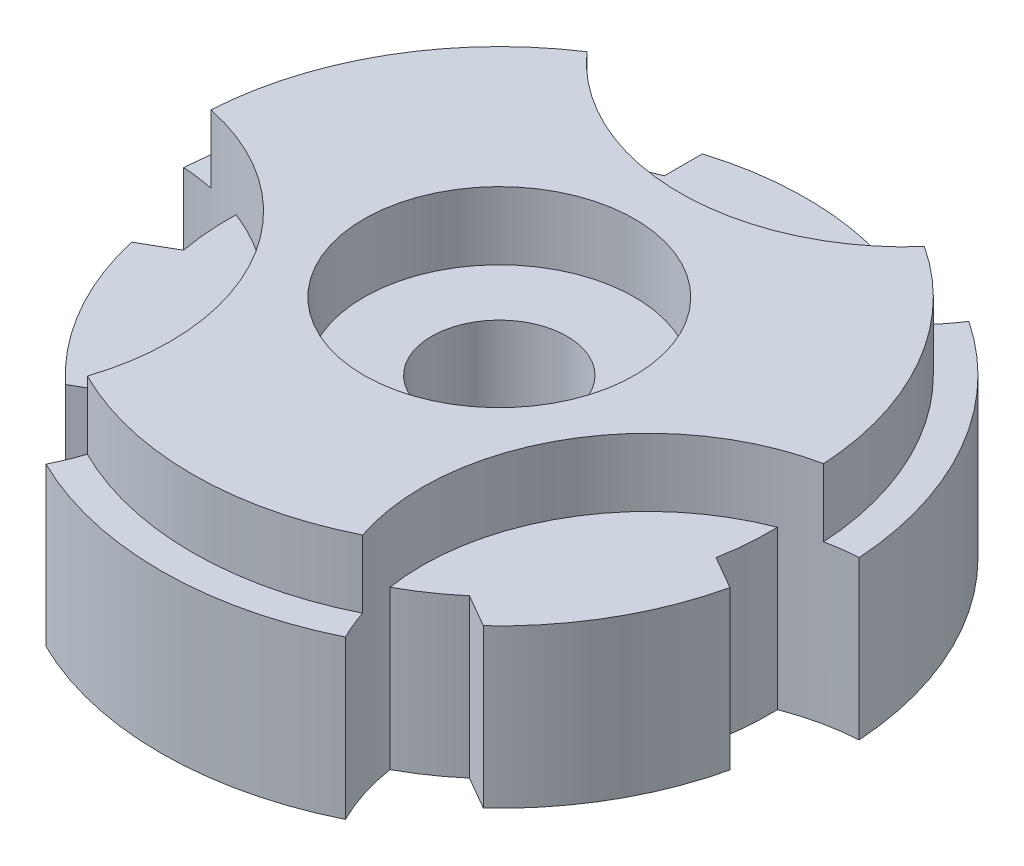
ISO-10303-21;
HEADER;
FILE_DESCRIPTION(('STEP AP214'),'2;1');
FILE_NAME('part.step','',(''),(''),'','','');
FILE_SCHEMA(('AUTOMOTIVE_DESIGN { 1 0 10303 214 1 1 1 1 }'));
ENDSEC;
DATA;
#1=APPLICATION_CONTEXT('core data for automotive mechanical design processes');
#2=APPLICATION_PROTOCOL_DEFINITION('international standard','automotive_design',2000,#1);
#3=PRODUCT_CONTEXT('',#1,'mechanical');
#4=PRODUCT('Part','Part','',(#3));
#5=PRODUCT_RELATED_PRODUCT_CATEGORY('part','',(#4));
#6=PRODUCT_DEFINITION_FORMATION('','',#4);
#7=PRODUCT_DEFINITION_CONTEXT('part definition',#1,'design');
#8=PRODUCT_DEFINITION('design','',#6,#7);
#9=PRODUCT_DEFINITION_SHAPE('','',#8);
#10=(LENGTH_UNIT() NAMED_UNIT(*) SI_UNIT(.MILLI.,.METRE.));
#11=(NAMED_UNIT(*) PLANE_ANGLE_UNIT() SI_UNIT($,.RADIAN.));
#12=(NAMED_UNIT(*) SI_UNIT($,.STERADIAN.) SOLID_ANGLE_UNIT());
#13=UNCERTAINTY_MEASURE_WITH_UNIT(LENGTH_MEASURE(1.E-05),#10,'distance_accuracy_value','');
#14=(GEOMETRIC_REPRESENTATION_CONTEXT(3) GLOBAL_UNCERTAINTY_ASSIGNED_CONTEXT((#13)) GLOBAL_UNIT_ASSIGNED_CONTEXT((#10,
#11,#12)) REPRESENTATION_CONTEXT('',''));
#15=CARTESIAN_POINT('',(0.,0.,0.));
#16=DIRECTION('',(0.,0.,1.));
#17=DIRECTION('',(1.,0.,0.));
#18=AXIS2_PLACEMENT_3D('',#15,#16,#17);
#19=CARTESIAN_POINT('',(-38.9711431702998,35.,22.4999999999999));
#20=DIRECTION('',(0.,1.,0.));
#21=DIRECTION('',(0.,0.,1.));
#22=AXIS2_PLACEMENT_3D('',#19,#20,#21);
#23=PLANE('',#22);
#24=CARTESIAN_POINT('',(-77.9422863405843,35.,44.9999999999979));
#25=DIRECTION('',(0.,-1.,0.));
#26=DIRECTION('',(0.,0.,1.));
#27=AXIS2_PLACEMENT_3D('',#24,#25,#26);
#28=CIRCLE('',#27,50.);
#29=CARTESIAN_POINT('',(-59.977004664239,35.,-1.66099714203543));
#30=VERTEX_POINT('',#29);
#31=CARTESIAN_POINT('',(-28.5500366115037,35.,52.7721082531464));
#32=VERTEX_POINT('',#31);
#33=EDGE_CURVE('E11',#30,#32,#28,.T.);
#34=ORIENTED_EDGE('',*,*,#33,.F.);
#35=CARTESIAN_POINT('',(0.,35.,0.));
#36=DIRECTION('',(0.,-1.,0.));
#37=DIRECTION('',(0.,0.,-1.));
#38=AXIS2_PLACEMENT_3D('',#35,#36,#37);
#39=CIRCLE('',#38,60.);
#40=CARTESIAN_POINT('',(-58.9897948556635,35.,10.9637631717732));
#41=VERTEX_POINT('',#40);
#42=EDGE_CURVE('E300',#41,#30,#39,.T.);
#43=ORIENTED_EDGE('',*,*,#42,.F.);
#44=DIRECTION('',(0.866025403784438,0.,-0.500000000000002));
#45=VECTOR('',#44,1.);
#46=CARTESIAN_POINT('',(-58.9897948556635,35.,10.9637631717732));
#47=LINE('',#46,#45);
#48=CARTESIAN_POINT('',(-66.2849891178811,35.,15.1756455428552));
#49=VERTEX_POINT('',#48);
#50=EDGE_CURVE('E291',#49,#41,#47,.T.);
#51=ORIENTED_EDGE('',*,*,#50,.F.);
#52=CARTESIAN_POINT('',(0.,35.,0.));
#53=DIRECTION('',(0.,-1.,0.));
#54=DIRECTION('',(0.,0.,-1.));
#55=AXIS2_PLACEMENT_3D('',#52,#53,#54);
#56=CIRCLE('',#55,68.);
#57=CARTESIAN_POINT('',(-46.2849891178811,35.,49.8166616942327));
#58=VERTEX_POINT('',#57);
#59=EDGE_CURVE('E287',#58,#49,#56,.T.);
#60=ORIENTED_EDGE('',*,*,#59,.F.);
#61=DIRECTION('',(-0.866025403784437,0.,0.500000000000002));
#62=VECTOR('',#61,1.);
#63=CARTESIAN_POINT('',(-38.9897948556635,35.,45.6047793231507));
#64=LINE('',#63,#62);
#65=CARTESIAN_POINT('',(-38.9897948556635,35.,45.6047793231508));
#66=VERTEX_POINT('',#65);
#67=EDGE_CURVE('E290',#66,#58,#64,.T.);
#68=ORIENTED_EDGE('',*,*,#67,.F.);
#69=CARTESIAN_POINT('',(0.,35.,0.));
#70=DIRECTION('',(0.,-1.,0.));
#71=DIRECTION('',(0.,0.,-1.));
#72=AXIS2_PLACEMENT_3D('',#69,#70,#71);
#73=CIRCLE('',#72,60.);
#74=EDGE_CURVE('E282',#32,#66,#73,.T.);
#75=ORIENTED_EDGE('',*,*,#74,.F.);
#76=EDGE_LOOP('',(#34,#43,#51,#60,#68,#75));
#77=FACE_BOUND('',#76,.T.);
#78=ADVANCED_FACE('F44',(#77),#23,.T.);
#79=CARTESIAN_POINT('',(0.,35.,0.));
#80=DIRECTION('',(0.,1.,0.));
#81=DIRECTION('',(0.,0.,1.));
#82=AXIS2_PLACEMENT_3D('',#79,#80,#81);
#83=CIRCLE('',#82,68.);
#84=CARTESIAN_POINT('',(-37.386628625753,35.,-56.8000000000003));
#85=VERTEX_POINT('',#84);
#86=CARTESIAN_POINT('',(-67.8835572478328,35.,-3.97777015175703));
#87=VERTEX_POINT('',#86);
#88=EDGE_CURVE('E263',#85,#87,#83,.T.);
#89=ORIENTED_EDGE('',*,*,#88,.F.);
#90=CARTESIAN_POINT('',(5.89805981832114E-13,35.,-90.));
#91=DIRECTION('',(0.,-1.,0.));
#92=DIRECTION('',(0.,0.,1.));
#93=AXIS2_PLACEMENT_3D('',#90,#91,#92);
#94=CIRCLE('',#93,50.);
#95=CARTESIAN_POINT('',(-41.6664351845418,35.,-62.3611111111114));
#96=VERTEX_POINT('',#95);
#97=EDGE_CURVE('E404',#85,#96,#94,.T.);
#98=ORIENTED_EDGE('',*,*,#97,.T.);
#99=CARTESIAN_POINT('',(0.,35.,0.));
#100=DIRECTION('',(0.,1.,0.));
#101=DIRECTION('',(0.,0.,1.));
#102=AXIS2_PLACEMENT_3D('',#99,#100,#101);
#103=CIRCLE('',#102,75.);
#104=CARTESIAN_POINT('',(-74.8395240227173,35.,-4.90363579939592));
#105=VERTEX_POINT('',#104);
#106=EDGE_CURVE('E410',#96,#105,#103,.T.);
#107=ORIENTED_EDGE('',*,*,#106,.T.);
#108=CARTESIAN_POINT('',(-77.9422863405996,35.,44.9999999999999));
#109=DIRECTION('',(0.,-1.,0.));
#110=DIRECTION('',(0.,0.,1.));
#111=AXIS2_PLACEMENT_3D('',#108,#109,#110);
#112=CIRCLE('',#111,50.);
#113=EDGE_CURVE('E67',#105,#87,#112,.T.);
#114=ORIENTED_EDGE('',*,*,#113,.T.);
#115=EDGE_LOOP('',(#89,#98,#107,#114));
#116=FACE_BOUND('',#115,.T.);
#117=ADVANCED_FACE('F535',(#116),#23,.T.);
#118=CARTESIAN_POINT('',(0.,35.,-90.));
#119=DIRECTION('',(0.,-1.,0.));
#120=DIRECTION('',(0.,0.,1.));
#121=AXIS2_PLACEMENT_3D('',#118,#119,#120);
#122=CIRCLE('',#121,50.);
#123=CARTESIAN_POINT('',(31.4269680527358,35.,-51.1111111111109));
#124=VERTEX_POINT('',#123);
#125=CARTESIAN_POINT('',(-31.4269680527351,35.,-51.1111111111113));
#126=VERTEX_POINT('',#125);
#127=EDGE_CURVE('E53',#124,#126,#122,.T.);
#128=ORIENTED_EDGE('',*,*,#127,.F.);
#129=CARTESIAN_POINT('',(0.,35.,0.));
#130=DIRECTION('',(0.,-1.,0.));
#131=DIRECTION('',(0.,0.,-1.));
#132=AXIS2_PLACEMENT_3D('',#129,#130,#131);
#133=CIRCLE('',#132,60.);
#134=CARTESIAN_POINT('',(19.9999999999999,35.,-56.5685424949238));
#135=VERTEX_POINT('',#134);
#136=EDGE_CURVE('E309',#135,#124,#133,.T.);
#137=ORIENTED_EDGE('',*,*,#136,.F.);
#138=DIRECTION('',(0.,0.,1.));
#139=VECTOR('',#138,1.);
#140=CARTESIAN_POINT('',(19.9999999999999,35.,-56.5685424949238));
#141=LINE('',#140,#139);
#142=CARTESIAN_POINT('',(19.9999999999999,35.,-64.9923072370877));
#143=VERTEX_POINT('',#142);
#144=EDGE_CURVE('E308',#143,#135,#141,.T.);
#145=ORIENTED_EDGE('',*,*,#144,.F.);
#146=CARTESIAN_POINT('',(0.,35.,0.));
#147=DIRECTION('',(0.,-1.,0.));
#148=DIRECTION('',(0.,0.,-1.));
#149=AXIS2_PLACEMENT_3D('',#146,#147,#148);
#150=CIRCLE('',#149,68.);
#151=CARTESIAN_POINT('',(-20.0000000000001,35.,-64.9923072370877));
#152=VERTEX_POINT('',#151);
#153=EDGE_CURVE('E301',#152,#143,#150,.T.);
#154=ORIENTED_EDGE('',*,*,#153,.F.);
#155=DIRECTION('',(0.,0.,-1.));
#156=VECTOR('',#155,1.);
#157=CARTESIAN_POINT('',(-20.0000000000001,35.,-56.5685424949238));
#158=LINE('',#157,#156);
#159=CARTESIAN_POINT('',(-20.0000000000002,35.,-56.5685424949238));
#160=VERTEX_POINT('',#159);
#161=EDGE_CURVE('E299',#160,#152,#158,.T.);
#162=ORIENTED_EDGE('',*,*,#161,.F.);
#163=EDGE_CURVE('E296',#126,#160,#39,.T.);
#164=ORIENTED_EDGE('',*,*,#163,.F.);
#165=EDGE_LOOP('',(#128,#137,#145,#154,#162,#164));
#166=FACE_BOUND('',#165,.T.);
#167=ADVANCED_FACE('F539',(#166),#23,.T.);
#168=CARTESIAN_POINT('',(0.,35.,0.));
#169=DIRECTION('',(0.,1.,0.));
#170=DIRECTION('',(0.,0.,1.));
#171=AXIS2_PLACEMENT_3D('',#168,#169,#170);
#172=CIRCLE('',#171,68.);
#173=CARTESIAN_POINT('',(67.8835572478346,35.,-3.97777015175745));
#174=VERTEX_POINT('',#173);
#175=CARTESIAN_POINT('',(37.3866286257538,35.,-56.7999999999997));
#176=VERTEX_POINT('',#175);
#177=EDGE_CURVE('E449',#174,#176,#172,.T.);
#178=ORIENTED_EDGE('',*,*,#177,.F.);
#179=CARTESIAN_POINT('',(77.9422863405996,35.,44.9999999999998));
#180=DIRECTION('',(0.,-1.,0.));
#181=DIRECTION('',(0.,0.,1.));
#182=AXIS2_PLACEMENT_3D('',#179,#180,#181);
#183=CIRCLE('',#182,50.);
#184=CARTESIAN_POINT('',(74.8395240227173,35.,-4.90363579939593));
#185=VERTEX_POINT('',#184);
#186=EDGE_CURVE('E399',#174,#185,#183,.T.);
#187=ORIENTED_EDGE('',*,*,#186,.T.);
#188=CARTESIAN_POINT('',(0.,35.,0.));
#189=DIRECTION('',(0.,1.,0.));
#190=DIRECTION('',(0.,0.,1.));
#191=AXIS2_PLACEMENT_3D('',#188,#189,#190);
#192=CIRCLE('',#191,75.);
#193=CARTESIAN_POINT('',(41.6664351845426,35.,-62.3611111111108));
#194=VERTEX_POINT('',#193);
#195=EDGE_CURVE('E405',#185,#194,#192,.T.);
#196=ORIENTED_EDGE('',*,*,#195,.T.);
#197=EDGE_CURVE('E403',#194,#176,#94,.T.);
#198=ORIENTED_EDGE('',*,*,#197,.T.);
#199=EDGE_LOOP('',(#178,#187,#196,#198));
#200=FACE_BOUND('',#199,.T.);
#201=ADVANCED_FACE('F471',(#200),#23,.T.);
#202=CARTESIAN_POINT('',(77.9422863406052,35.,44.9999999999858));
#203=DIRECTION('',(0.,-1.,0.));
#204=DIRECTION('',(0.,0.,1.));
#205=AXIS2_PLACEMENT_3D('',#202,#203,#204);
#206=CIRCLE('',#205,50.);
#207=CARTESIAN_POINT('',(28.5500366115037,35.,52.7721082531463));
#208=VERTEX_POINT('',#207);
#209=CARTESIAN_POINT('',(59.977004664239,35.,-1.66099714203546));
#210=VERTEX_POINT('',#209);
#211=EDGE_CURVE('E442',#208,#210,#206,.T.);
#212=ORIENTED_EDGE('',*,*,#211,.F.);
#213=CARTESIAN_POINT('',(38.9897948556637,35.,45.6047793231506));
#214=VERTEX_POINT('',#213);
#215=EDGE_CURVE('E283',#214,#208,#73,.T.);
#216=ORIENTED_EDGE('',*,*,#215,.F.);
#217=DIRECTION('',(-0.86602540378444,0.,-0.499999999999997));
#218=VECTOR('',#217,1.);
#219=CARTESIAN_POINT('',(38.9897948556637,35.,45.6047793231506));
#220=LINE('',#219,#218);
#221=CARTESIAN_POINT('',(46.2849891178813,35.,49.8166616942325));
#222=VERTEX_POINT('',#221);
#223=EDGE_CURVE('E276',#222,#214,#220,.T.);
#224=ORIENTED_EDGE('',*,*,#223,.F.);
#225=CARTESIAN_POINT('',(0.,35.,0.));
#226=DIRECTION('',(0.,-1.,0.));
#227=DIRECTION('',(0.,0.,-1.));
#228=AXIS2_PLACEMENT_3D('',#225,#226,#227);
#229=CIRCLE('',#228,68.);
#230=CARTESIAN_POINT('',(66.2849891178812,35.,15.1756455428549));
#231=VERTEX_POINT('',#230);
#232=EDGE_CURVE('E277',#231,#222,#229,.T.);
#233=ORIENTED_EDGE('',*,*,#232,.F.);
#234=DIRECTION('',(0.866025403784439,0.,0.499999999999999));
#235=VECTOR('',#234,1.);
#236=CARTESIAN_POINT('',(58.9897948556636,35.,10.963763171773));
#237=LINE('',#236,#235);
#238=CARTESIAN_POINT('',(58.9897948556636,35.,10.963763171773));
#239=VERTEX_POINT('',#238);
#240=EDGE_CURVE('E311',#239,#231,#237,.T.);
#241=ORIENTED_EDGE('',*,*,#240,.F.);
#242=EDGE_CURVE('E310',#210,#239,#133,.T.);
#243=ORIENTED_EDGE('',*,*,#242,.F.);
#244=EDGE_LOOP('',(#212,#216,#224,#233,#241,#243));
#245=FACE_BOUND('',#244,.T.);
#246=ADVANCED_FACE('F544',(#245),#23,.T.);
#247=CARTESIAN_POINT('',(-77.9422863405996,35.,44.9999999999999));
#248=DIRECTION('',(0.,-1.,0.));
#249=DIRECTION('',(0.,0.,-1.));
#250=AXIS2_PLACEMENT_3D('',#247,#248,#249);
#251=CYLINDRICAL_SURFACE('',#250,50.);
#252=CARTESIAN_POINT('',(-30.4969286220795,35.,60.7777701517569));
#253=VERTEX_POINT('',#252);
#254=CARTESIAN_POINT('',(-33.1730888381753,35.,67.2647469105068));
#255=VERTEX_POINT('',#254);
#256=EDGE_CURVE('E266',#253,#255,#112,.T.);
#257=ORIENTED_EDGE('',*,*,#256,.F.);
#258=DIRECTION('',(0.,-1.,0.));
#259=VECTOR('',#258,1.);
#260=CARTESIAN_POINT('',(-30.496928622067,50.,60.7777701517631));
#261=LINE('',#260,#259);
#262=CARTESIAN_POINT('',(-30.496928622067,50.,60.7777701517631));
#263=VERTEX_POINT('',#262);
#264=EDGE_CURVE('E246',#263,#253,#261,.T.);
#265=ORIENTED_EDGE('',*,*,#264,.F.);
#266=CARTESIAN_POINT('',(-77.9422863405843,50.,44.9999999999979));
#267=DIRECTION('',(0.,-1.,0.));
#268=DIRECTION('',(0.,0.,1.));
#269=AXIS2_PLACEMENT_3D('',#266,#267,#268);
#270=CIRCLE('',#269,50.);
#271=CARTESIAN_POINT('',(-67.8835572478325,50.,-3.97777015176211));
#272=VERTEX_POINT('',#271);
#273=EDGE_CURVE('E255',#272,#263,#270,.T.);
#274=ORIENTED_EDGE('',*,*,#273,.F.);
#275=DIRECTION('',(0.,-1.,0.));
#276=VECTOR('',#275,1.);
#277=CARTESIAN_POINT('',(-67.8835572478325,50.,-3.97777015176211));
#278=LINE('',#277,#276);
#279=EDGE_CURVE('E454',#272,#87,#278,.T.);
#280=ORIENTED_EDGE('',*,*,#279,.T.);
#281=ORIENTED_EDGE('',*,*,#113,.F.);
#282=DIRECTION('',(0.,-1.,0.));
#283=VECTOR('',#282,1.);
#284=CARTESIAN_POINT('',(-74.8395240227173,35.,-4.90363579939592));
#285=LINE('',#284,#283);
#286=CARTESIAN_POINT('',(-74.8395240227173,0.,-4.90363579939592));
#287=VERTEX_POINT('',#286);
#288=EDGE_CURVE('E408',#105,#287,#285,.T.);
#289=ORIENTED_EDGE('',*,*,#288,.T.);
#290=CARTESIAN_POINT('',(-77.9422863405996,0.,44.9999999999999));
#291=DIRECTION('',(0.,-1.,0.));
#292=DIRECTION('',(0.,0.,1.));
#293=AXIS2_PLACEMENT_3D('',#290,#291,#292);
#294=CIRCLE('',#293,50.);
#295=CARTESIAN_POINT('',(-59.977004664239,0.,-1.66099714203543));
#296=VERTEX_POINT('',#295);
#297=EDGE_CURVE('E409',#287,#296,#294,.T.);
#298=ORIENTED_EDGE('',*,*,#297,.T.);
#299=DIRECTION('',(0.,-1.,0.));
#300=VECTOR('',#299,1.);
#301=CARTESIAN_POINT('',(-59.977004664239,17.5,-1.66099714203543));
#302=LINE('',#301,#300);
#303=EDGE_CURVE('E387',#296,#30,#302,.F.);
#304=ORIENTED_EDGE('',*,*,#303,.T.);
#305=ORIENTED_EDGE('',*,*,#33,.T.);
#306=DIRECTION('',(0.,-1.,0.));
#307=VECTOR('',#306,1.);
#308=CARTESIAN_POINT('',(-28.5500366115037,17.5,52.7721082531464));
#309=LINE('',#308,#307);
#310=CARTESIAN_POINT('',(-28.5500366115037,0.,52.7721082531464));
#311=VERTEX_POINT('',#310);
#312=EDGE_CURVE('E379',#32,#311,#309,.T.);
#313=ORIENTED_EDGE('',*,*,#312,.T.);
#314=CARTESIAN_POINT('',(-33.1730888381753,0.,67.2647469105068));
#315=VERTEX_POINT('',#314);
#316=EDGE_CURVE('E394',#311,#315,#294,.T.);
#317=ORIENTED_EDGE('',*,*,#316,.T.);
#318=DIRECTION('',(0.,-1.,0.));
#319=VECTOR('',#318,1.);
#320=CARTESIAN_POINT('',(-33.1730888381753,35.,67.2647469105068));
#321=LINE('',#320,#319);
#322=EDGE_CURVE('E47',#255,#315,#321,.T.);
#323=ORIENTED_EDGE('',*,*,#322,.F.);
#324=EDGE_LOOP('',(#257,#265,#274,#280,#281,#289,#298,#304,#305,#313,#317,#323));
#325=FACE_BOUND('',#324,.T.);
#326=ADVANCED_FACE('F50',(#325),#251,.F.);
#327=CARTESIAN_POINT('',(0.,35.,0.));
#328=DIRECTION('',(0.,-1.,0.));
#329=DIRECTION('',(0.,0.,-1.));
#330=AXIS2_PLACEMENT_3D('',#327,#328,#329);
#331=CYLINDRICAL_SURFACE('',#330,75.);
#332=CARTESIAN_POINT('',(0.,0.,0.));
#333=DIRECTION('',(0.,1.,0.));
#334=DIRECTION('',(0.,0.,1.));
#335=AXIS2_PLACEMENT_3D('',#332,#333,#334);
#336=CIRCLE('',#335,75.);
#337=CARTESIAN_POINT('',(33.1730888381753,0.,67.2647469105067));
#338=VERTEX_POINT('',#337);
#339=EDGE_CURVE('E415',#315,#338,#336,.T.);
#340=ORIENTED_EDGE('',*,*,#339,.T.);
#341=DIRECTION('',(0.,-1.,0.));
#342=VECTOR('',#341,1.);
#343=CARTESIAN_POINT('',(33.1730888381753,35.,67.2647469105067));
#344=LINE('',#343,#342);
#345=CARTESIAN_POINT('',(33.1730888381753,35.,67.2647469105067));
#346=VERTEX_POINT('',#345);
#347=EDGE_CURVE('E432',#346,#338,#344,.T.);
#348=ORIENTED_EDGE('',*,*,#347,.F.);
#349=CARTESIAN_POINT('',(0.,35.,0.));
#350=DIRECTION('',(0.,1.,0.));
#351=DIRECTION('',(0.,0.,1.));
#352=AXIS2_PLACEMENT_3D('',#349,#350,#351);
#353=CIRCLE('',#352,75.);
#354=EDGE_CURVE('E400',#255,#346,#353,.T.);
#355=ORIENTED_EDGE('',*,*,#354,.F.);
#356=ORIENTED_EDGE('',*,*,#322,.T.);
#357=EDGE_LOOP('',(#340,#348,#355,#356));
#358=FACE_BOUND('',#357,.T.);
#359=ADVANCED_FACE('F563',(#358),#331,.T.);
#360=CARTESIAN_POINT('',(77.9422863405996,35.,44.9999999999998));
#361=DIRECTION('',(0.,-1.,0.));
#362=DIRECTION('',(0.,0.,-1.));
#363=AXIS2_PLACEMENT_3D('',#360,#361,#362);
#364=CYLINDRICAL_SURFACE('',#363,50.);
#365=CARTESIAN_POINT('',(77.9422863405996,0.,44.9999999999998));
#366=DIRECTION('',(0.,-1.,0.));
#367=DIRECTION('',(0.,0.,1.));
#368=AXIS2_PLACEMENT_3D('',#365,#366,#367);
#369=CIRCLE('',#368,50.);
#370=CARTESIAN_POINT('',(28.5500366115037,0.,52.7721082531463));
#371=VERTEX_POINT('',#370);
#372=EDGE_CURVE('E412',#338,#371,#369,.T.);
#373=ORIENTED_EDGE('',*,*,#372,.T.);
#374=DIRECTION('',(0.,-1.,0.));
#375=VECTOR('',#374,1.);
#376=CARTESIAN_POINT('',(28.5500366115037,17.5,52.7721082531463));
#377=LINE('',#376,#375);
#378=EDGE_CURVE('E352',#371,#208,#377,.F.);
#379=ORIENTED_EDGE('',*,*,#378,.T.);
#380=ORIENTED_EDGE('',*,*,#211,.T.);
#381=DIRECTION('',(0.,-1.,0.));
#382=VECTOR('',#381,1.);
#383=CARTESIAN_POINT('',(59.977004664239,17.5,-1.66099714203546));
#384=LINE('',#383,#382);
#385=CARTESIAN_POINT('',(59.977004664239,0.,-1.66099714203546));
#386=VERTEX_POINT('',#385);
#387=EDGE_CURVE('E395',#210,#386,#384,.T.);
#388=ORIENTED_EDGE('',*,*,#387,.T.);
#389=CARTESIAN_POINT('',(74.8395240227173,0.,-4.90363579939593));
#390=VERTEX_POINT('',#389);
#391=EDGE_CURVE('E414',#386,#390,#369,.T.);
#392=ORIENTED_EDGE('',*,*,#391,.T.);
#393=DIRECTION('',(0.,-1.,0.));
#394=VECTOR('',#393,1.);
#395=CARTESIAN_POINT('',(74.8395240227173,35.,-4.90363579939593));
#396=LINE('',#395,#394);
#397=EDGE_CURVE('E435',#185,#390,#396,.T.);
#398=ORIENTED_EDGE('',*,*,#397,.F.);
#399=ORIENTED_EDGE('',*,*,#186,.F.);
#400=DIRECTION('',(0.,-1.,0.));
#401=VECTOR('',#400,1.);
#402=CARTESIAN_POINT('',(67.883557247832,50.,-3.9777701517698));
#403=LINE('',#402,#401);
#404=CARTESIAN_POINT('',(67.883557247832,50.,-3.9777701517698));
#405=VERTEX_POINT('',#404);
#406=EDGE_CURVE('E275',#405,#174,#403,.T.);
#407=ORIENTED_EDGE('',*,*,#406,.F.);
#408=CARTESIAN_POINT('',(77.9422863406052,50.,44.9999999999858));
#409=DIRECTION('',(0.,-1.,0.));
#410=DIRECTION('',(0.,0.,1.));
#411=AXIS2_PLACEMENT_3D('',#408,#409,#410);
#412=CIRCLE('',#411,50.);
#413=CARTESIAN_POINT('',(30.4969286220884,50.,60.7777701517524));
#414=VERTEX_POINT('',#413);
#415=EDGE_CURVE('E251',#414,#405,#412,.T.);
#416=ORIENTED_EDGE('',*,*,#415,.F.);
#417=DIRECTION('',(0.,-1.,0.));
#418=VECTOR('',#417,1.);
#419=CARTESIAN_POINT('',(30.4969286220884,50.,60.7777701517524));
#420=LINE('',#419,#418);
#421=CARTESIAN_POINT('',(30.4969286220884,35.,60.7777701517524));
#422=VERTEX_POINT('',#421);
#423=EDGE_CURVE('E247',#414,#422,#420,.T.);
#424=ORIENTED_EDGE('',*,*,#423,.T.);
#425=EDGE_CURVE('E397',#346,#422,#183,.T.);
#426=ORIENTED_EDGE('',*,*,#425,.F.);
#427=ORIENTED_EDGE('',*,*,#347,.T.);
#428=EDGE_LOOP('',(#373,#379,#380,#388,#392,#398,#399,#407,#416,#424,#426,#427));
#429=FACE_BOUND('',#428,.T.);
#430=ADVANCED_FACE('F469',(#429),#364,.F.);
#431=CARTESIAN_POINT('',(0.,35.,0.));
#432=DIRECTION('',(0.,-1.,0.));
#433=DIRECTION('',(0.,0.,-1.));
#434=AXIS2_PLACEMENT_3D('',#431,#432,#433);
#435=CYLINDRICAL_SURFACE('',#434,75.);
#436=CARTESIAN_POINT('',(0.,0.,0.));
#437=DIRECTION('',(0.,1.,0.));
#438=DIRECTION('',(0.,0.,1.));
#439=AXIS2_PLACEMENT_3D('',#436,#437,#438);
#440=CIRCLE('',#439,75.);
#441=CARTESIAN_POINT('',(41.6664351845426,0.,-62.3611111111108));
#442=VERTEX_POINT('',#441);
#443=EDGE_CURVE('E417',#390,#442,#440,.T.);
#444=ORIENTED_EDGE('',*,*,#443,.T.);
#445=DIRECTION('',(0.,-1.,0.));
#446=VECTOR('',#445,1.);
#447=CARTESIAN_POINT('',(41.6664351845426,35.,-62.3611111111108));
#448=LINE('',#447,#446);
#449=EDGE_CURVE('E427',#194,#442,#448,.T.);
#450=ORIENTED_EDGE('',*,*,#449,.F.);
#451=ORIENTED_EDGE('',*,*,#195,.F.);
#452=ORIENTED_EDGE('',*,*,#397,.T.);
#453=EDGE_LOOP('',(#444,#450,#451,#452));
#454=FACE_BOUND('',#453,.T.);
#455=ADVANCED_FACE('F588',(#454),#435,.T.);
#456=CARTESIAN_POINT('',(5.89805981832114E-13,35.,-90.));
#457=DIRECTION('',(0.,-1.,0.));
#458=DIRECTION('',(0.,0.,-1.));
#459=AXIS2_PLACEMENT_3D('',#456,#457,#458);
#460=CYLINDRICAL_SURFACE('',#459,50.);
#461=ORIENTED_EDGE('',*,*,#97,.F.);
#462=DIRECTION('',(0.,-1.,0.));
#463=VECTOR('',#462,1.);
#464=CARTESIAN_POINT('',(-37.3866286257533,50.,-56.8));
#465=LINE('',#464,#463);
#466=CARTESIAN_POINT('',(-37.3866286257533,50.,-56.8));
#467=VERTEX_POINT('',#466);
#468=EDGE_CURVE('E457',#467,#85,#465,.T.);
#469=ORIENTED_EDGE('',*,*,#468,.F.);
#470=CARTESIAN_POINT('',(0.,50.,-90.));
#471=DIRECTION('',(0.,-1.,0.));
#472=DIRECTION('',(0.,0.,1.));
#473=AXIS2_PLACEMENT_3D('',#470,#471,#472);
#474=CIRCLE('',#473,50.);
#475=CARTESIAN_POINT('',(37.3866286257533,50.,-56.8));
#476=VERTEX_POINT('',#475);
#477=EDGE_CURVE('E485',#476,#467,#474,.T.);
#478=ORIENTED_EDGE('',*,*,#477,.F.);
#479=DIRECTION('',(0.,-1.,0.));
#480=VECTOR('',#479,1.);
#481=CARTESIAN_POINT('',(37.3866286257533,50.,-56.8));
#482=LINE('',#481,#480);
#483=EDGE_CURVE('E459',#476,#176,#482,.T.);
#484=ORIENTED_EDGE('',*,*,#483,.T.);
#485=ORIENTED_EDGE('',*,*,#197,.F.);
#486=ORIENTED_EDGE('',*,*,#449,.T.);
#487=CARTESIAN_POINT('',(5.89805981832114E-13,0.,-90.));
#488=DIRECTION('',(0.,-1.,0.));
#489=DIRECTION('',(0.,0.,1.));
#490=AXIS2_PLACEMENT_3D('',#487,#488,#489);
#491=CIRCLE('',#490,50.);
#492=CARTESIAN_POINT('',(31.4269680527358,0.,-51.1111111111109));
#493=VERTEX_POINT('',#492);
#494=EDGE_CURVE('E419',#442,#493,#491,.T.);
#495=ORIENTED_EDGE('',*,*,#494,.T.);
#496=DIRECTION('',(0.,-1.,0.));
#497=VECTOR('',#496,1.);
#498=CARTESIAN_POINT('',(31.4269680527358,17.5,-51.1111111111109));
#499=LINE('',#498,#497);
#500=EDGE_CURVE('E386',#493,#124,#499,.F.);
#501=ORIENTED_EDGE('',*,*,#500,.T.);
#502=ORIENTED_EDGE('',*,*,#127,.T.);
#503=DIRECTION('',(0.,-1.,0.));
#504=VECTOR('',#503,1.);
#505=CARTESIAN_POINT('',(-31.4269680527351,17.5,-51.1111111111113));
#506=LINE('',#505,#504);
#507=CARTESIAN_POINT('',(-31.4269680527351,0.,-51.1111111111113));
#508=VERTEX_POINT('',#507);
#509=EDGE_CURVE('E382',#126,#508,#506,.T.);
#510=ORIENTED_EDGE('',*,*,#509,.T.);
#511=CARTESIAN_POINT('',(-41.6664351845418,0.,-62.3611111111114));
#512=VERTEX_POINT('',#511);
#513=EDGE_CURVE('E420',#508,#512,#491,.T.);
#514=ORIENTED_EDGE('',*,*,#513,.T.);
#515=DIRECTION('',(0.,-1.,0.));
#516=VECTOR('',#515,1.);
#517=CARTESIAN_POINT('',(-41.6664351845418,35.,-62.3611111111114));
#518=LINE('',#517,#516);
#519=EDGE_CURVE('E426',#96,#512,#518,.T.);
#520=ORIENTED_EDGE('',*,*,#519,.F.);
#521=EDGE_LOOP('',(#461,#469,#478,#484,#485,#486,#495,#501,#502,#510,#514,#520));
#522=FACE_BOUND('',#521,.T.);
#523=ADVANCED_FACE('F476',(#522),#460,.F.);
#524=CARTESIAN_POINT('',(0.,35.,0.));
#525=DIRECTION('',(0.,-1.,0.));
#526=DIRECTION('',(0.,0.,-1.));
#527=AXIS2_PLACEMENT_3D('',#524,#525,#526);
#528=CYLINDRICAL_SURFACE('',#527,75.);
#529=CARTESIAN_POINT('',(0.,0.,0.));
#530=DIRECTION('',(0.,1.,0.));
#531=DIRECTION('',(0.,0.,1.));
#532=AXIS2_PLACEMENT_3D('',#529,#530,#531);
#533=CIRCLE('',#532,75.);
#534=EDGE_CURVE('E425',#512,#287,#533,.T.);
#535=ORIENTED_EDGE('',*,*,#534,.T.);
#536=ORIENTED_EDGE('',*,*,#288,.F.);
#537=ORIENTED_EDGE('',*,*,#106,.F.);
#538=ORIENTED_EDGE('',*,*,#519,.T.);
#539=EDGE_LOOP('',(#535,#536,#537,#538));
#540=FACE_BOUND('',#539,.T.);
#541=ADVANCED_FACE('F542',(#540),#528,.T.);
#542=CARTESIAN_POINT('',(0.,35.,0.));
#543=DIRECTION('',(0.,1.,0.));
#544=DIRECTION('',(0.,0.,1.));
#545=AXIS2_PLACEMENT_3D('',#542,#543,#544);
#546=CIRCLE('',#545,68.);
#547=EDGE_CURVE('E65',#253,#422,#546,.T.);
#548=ORIENTED_EDGE('',*,*,#547,.F.);
#549=ORIENTED_EDGE('',*,*,#256,.T.);
#550=ORIENTED_EDGE('',*,*,#354,.T.);
#551=ORIENTED_EDGE('',*,*,#425,.T.);
#552=EDGE_LOOP('',(#548,#549,#550,#551));
#553=FACE_BOUND('',#552,.T.);
#554=ADVANCED_FACE('F532',(#553),#23,.T.);
#555=CARTESIAN_POINT('',(-38.9711431702998,0.,22.4999999999999));
#556=DIRECTION('',(0.,1.,0.));
#557=DIRECTION('',(0.,0.,1.));
#558=AXIS2_PLACEMENT_3D('',#555,#556,#557);
#559=PLANE('',#558);
#560=CARTESIAN_POINT('',(0.,0.,0.));
#561=DIRECTION('',(0.,1.,0.));
#562=DIRECTION('',(0.,0.,1.));
#563=AXIS2_PLACEMENT_3D('',#560,#561,#562);
#564=CIRCLE('',#563,15.);
#565=CARTESIAN_POINT('',(0.,0.,15.));
#566=VERTEX_POINT('',#565);
#567=EDGE_CURVE('E495',#566,#566,#564,.T.);
#568=ORIENTED_EDGE('',*,*,#567,.T.);
#569=EDGE_LOOP('',(#568));
#570=FACE_BOUND('',#569,.T.);
#571=ORIENTED_EDGE('',*,*,#316,.F.);
#572=CARTESIAN_POINT('',(0.,0.,0.));
#573=DIRECTION('',(0.,-1.,0.));
#574=DIRECTION('',(0.,0.,-1.));
#575=AXIS2_PLACEMENT_3D('',#572,#573,#574);
#576=CIRCLE('',#575,60.);
#577=CARTESIAN_POINT('',(-38.9897948556635,0.,45.6047793231508));
#578=VERTEX_POINT('',#577);
#579=EDGE_CURVE('E317',#311,#578,#576,.T.);
#580=ORIENTED_EDGE('',*,*,#579,.T.);
#581=DIRECTION('',(-0.866025403784437,0.,0.500000000000002));
#582=VECTOR('',#581,1.);
#583=CARTESIAN_POINT('',(-38.9897948556635,0.,45.6047793231507));
#584=LINE('',#583,#582);
#585=CARTESIAN_POINT('',(-46.2849891178811,0.,49.8166616942327));
#586=VERTEX_POINT('',#585);
#587=EDGE_CURVE('E323',#578,#586,#584,.T.);
#588=ORIENTED_EDGE('',*,*,#587,.T.);
#589=CARTESIAN_POINT('',(0.,0.,0.));
#590=DIRECTION('',(0.,-1.,0.));
#591=DIRECTION('',(0.,0.,-1.));
#592=AXIS2_PLACEMENT_3D('',#589,#590,#591);
#593=CIRCLE('',#592,68.);
#594=CARTESIAN_POINT('',(-66.2849891178811,0.,15.1756455428552));
#595=VERTEX_POINT('',#594);
#596=EDGE_CURVE('E326',#586,#595,#593,.T.);
#597=ORIENTED_EDGE('',*,*,#596,.T.);
#598=DIRECTION('',(0.866025403784438,0.,-0.500000000000002));
#599=VECTOR('',#598,1.);
#600=CARTESIAN_POINT('',(-58.9897948556635,0.,10.9637631717732));
#601=LINE('',#600,#599);
#602=CARTESIAN_POINT('',(-58.9897948556635,0.,10.9637631717732));
#603=VERTEX_POINT('',#602);
#604=EDGE_CURVE('E328',#595,#603,#601,.T.);
#605=ORIENTED_EDGE('',*,*,#604,.T.);
#606=CARTESIAN_POINT('',(0.,0.,0.));
#607=DIRECTION('',(0.,-1.,0.));
#608=DIRECTION('',(0.,0.,-1.));
#609=AXIS2_PLACEMENT_3D('',#606,#607,#608);
#610=CIRCLE('',#609,60.);
#611=EDGE_CURVE('E334',#603,#296,#610,.T.);
#612=ORIENTED_EDGE('',*,*,#611,.T.);
#613=ORIENTED_EDGE('',*,*,#297,.F.);
#614=ORIENTED_EDGE('',*,*,#534,.F.);
#615=ORIENTED_EDGE('',*,*,#513,.F.);
#616=CARTESIAN_POINT('',(-20.0000000000002,0.,-56.5685424949238));
#617=VERTEX_POINT('',#616);
#618=EDGE_CURVE('E335',#508,#617,#610,.T.);
#619=ORIENTED_EDGE('',*,*,#618,.T.);
#620=DIRECTION('',(0.,0.,-1.));
#621=VECTOR('',#620,1.);
#622=CARTESIAN_POINT('',(-20.0000000000001,0.,-56.5685424949238));
#623=LINE('',#622,#621);
#624=CARTESIAN_POINT('',(-20.0000000000001,0.,-64.9923072370877));
#625=VERTEX_POINT('',#624);
#626=EDGE_CURVE('E336',#617,#625,#623,.T.);
#627=ORIENTED_EDGE('',*,*,#626,.T.);
#628=CARTESIAN_POINT('',(0.,0.,0.));
#629=DIRECTION('',(0.,-1.,0.));
#630=DIRECTION('',(0.,0.,-1.));
#631=AXIS2_PLACEMENT_3D('',#628,#629,#630);
#632=CIRCLE('',#631,68.);
#633=CARTESIAN_POINT('',(19.9999999999999,0.,-64.9923072370877));
#634=VERTEX_POINT('',#633);
#635=EDGE_CURVE('E338',#625,#634,#632,.T.);
#636=ORIENTED_EDGE('',*,*,#635,.T.);
#637=DIRECTION('',(0.,0.,1.));
#638=VECTOR('',#637,1.);
#639=CARTESIAN_POINT('',(19.9999999999999,0.,-56.5685424949238));
#640=LINE('',#639,#638);
#641=CARTESIAN_POINT('',(19.9999999999999,0.,-56.5685424949238));
#642=VERTEX_POINT('',#641);
#643=EDGE_CURVE('E345',#634,#642,#640,.T.);
#644=ORIENTED_EDGE('',*,*,#643,.T.);
#645=CARTESIAN_POINT('',(0.,0.,0.));
#646=DIRECTION('',(0.,-1.,0.));
#647=DIRECTION('',(0.,0.,-1.));
#648=AXIS2_PLACEMENT_3D('',#645,#646,#647);
#649=CIRCLE('',#648,60.);
#650=EDGE_CURVE('E347',#642,#493,#649,.T.);
#651=ORIENTED_EDGE('',*,*,#650,.T.);
#652=ORIENTED_EDGE('',*,*,#494,.F.);
#653=ORIENTED_EDGE('',*,*,#443,.F.);
#654=ORIENTED_EDGE('',*,*,#391,.F.);
#655=CARTESIAN_POINT('',(58.9897948556636,0.,10.963763171773));
#656=VERTEX_POINT('',#655);
#657=EDGE_CURVE('E342',#386,#656,#649,.T.);
#658=ORIENTED_EDGE('',*,*,#657,.T.);
#659=DIRECTION('',(0.866025403784439,0.,0.499999999999999));
#660=VECTOR('',#659,1.);
#661=CARTESIAN_POINT('',(58.9897948556636,0.,10.963763171773));
#662=LINE('',#661,#660);
#663=CARTESIAN_POINT('',(66.2849891178812,0.,15.1756455428549));
#664=VERTEX_POINT('',#663);
#665=EDGE_CURVE('E278',#656,#664,#662,.T.);
#666=ORIENTED_EDGE('',*,*,#665,.T.);
#667=CARTESIAN_POINT('',(0.,0.,0.));
#668=DIRECTION('',(0.,-1.,0.));
#669=DIRECTION('',(0.,0.,-1.));
#670=AXIS2_PLACEMENT_3D('',#667,#668,#669);
#671=CIRCLE('',#670,68.);
#672=CARTESIAN_POINT('',(46.2849891178813,0.,49.8166616942325));
#673=VERTEX_POINT('',#672);
#674=EDGE_CURVE('E270',#664,#673,#671,.T.);
#675=ORIENTED_EDGE('',*,*,#674,.T.);
#676=DIRECTION('',(-0.86602540378444,0.,-0.499999999999997));
#677=VECTOR('',#676,1.);
#678=CARTESIAN_POINT('',(38.9897948556637,0.,45.6047793231506));
#679=LINE('',#678,#677);
#680=CARTESIAN_POINT('',(38.9897948556637,0.,45.6047793231506));
#681=VERTEX_POINT('',#680);
#682=EDGE_CURVE('E269',#673,#681,#679,.T.);
#683=ORIENTED_EDGE('',*,*,#682,.T.);
#684=EDGE_CURVE('E319',#681,#371,#576,.T.);
#685=ORIENTED_EDGE('',*,*,#684,.T.);
#686=ORIENTED_EDGE('',*,*,#372,.F.);
#687=ORIENTED_EDGE('',*,*,#339,.F.);
#688=EDGE_LOOP('',(#571,#580,#588,#597,#605,#612,#613,#614,#615,#619,#627,#636,#644,#651,#652,
#653,#654,#658,#666,#675,#683,#685,#686,#687));
#689=FACE_BOUND('',#688,.T.);
#690=ADVANCED_FACE('F501',(#570,#689),#559,.F.);
#691=CARTESIAN_POINT('',(19.9999999999999,35.,-56.5685424949238));
#692=DIRECTION('',(1.,0.,0.));
#693=DIRECTION('',(0.,0.,-1.));
#694=AXIS2_PLACEMENT_3D('',#691,#692,#693);
#695=PLANE('',#694);
#696=ORIENTED_EDGE('',*,*,#643,.F.);
#697=DIRECTION('',(0.,-1.,0.));
#698=VECTOR('',#697,1.);
#699=CARTESIAN_POINT('',(19.9999999999999,35.,-64.9923072370877));
#700=LINE('',#699,#698);
#701=EDGE_CURVE('E359',#143,#634,#700,.T.);
#702=ORIENTED_EDGE('',*,*,#701,.F.);
#703=ORIENTED_EDGE('',*,*,#144,.T.);
#704=DIRECTION('',(0.,-1.,0.));
#705=VECTOR('',#704,1.);
#706=CARTESIAN_POINT('',(19.9999999999999,35.,-56.5685424949238));
#707=LINE('',#706,#705);
#708=EDGE_CURVE('E360',#135,#642,#707,.T.);
#709=ORIENTED_EDGE('',*,*,#708,.T.);
#710=EDGE_LOOP('',(#696,#702,#703,#709));
#711=FACE_BOUND('',#710,.T.);
#712=ADVANCED_FACE('F552',(#711),#695,.T.);
#713=CARTESIAN_POINT('',(0.,35.,0.));
#714=DIRECTION('',(0.,-1.,0.));
#715=DIRECTION('',(0.,0.,-1.));
#716=AXIS2_PLACEMENT_3D('',#713,#714,#715);
#717=CYLINDRICAL_SURFACE('',#716,68.);
#718=ORIENTED_EDGE('',*,*,#635,.F.);
#719=DIRECTION('',(0.,-1.,0.));
#720=VECTOR('',#719,1.);
#721=CARTESIAN_POINT('',(-20.0000000000001,35.,-64.9923072370877));
#722=LINE('',#721,#720);
#723=EDGE_CURVE('E363',#152,#625,#722,.T.);
#724=ORIENTED_EDGE('',*,*,#723,.F.);
#725=ORIENTED_EDGE('',*,*,#153,.T.);
#726=ORIENTED_EDGE('',*,*,#701,.T.);
#727=EDGE_LOOP('',(#718,#724,#725,#726));
#728=FACE_BOUND('',#727,.T.);
#729=ADVANCED_FACE('F599',(#728),#717,.T.);
#730=CARTESIAN_POINT('',(-20.0000000000001,35.,-56.5685424949238));
#731=DIRECTION('',(-1.,0.,0.));
#732=DIRECTION('',(0.,0.,1.));
#733=AXIS2_PLACEMENT_3D('',#730,#731,#732);
#734=PLANE('',#733);
#735=ORIENTED_EDGE('',*,*,#626,.F.);
#736=DIRECTION('',(0.,-1.,0.));
#737=VECTOR('',#736,1.);
#738=CARTESIAN_POINT('',(-20.0000000000002,35.,-56.5685424949238));
#739=LINE('',#738,#737);
#740=EDGE_CURVE('E361',#160,#617,#739,.T.);
#741=ORIENTED_EDGE('',*,*,#740,.F.);
#742=ORIENTED_EDGE('',*,*,#161,.T.);
#743=ORIENTED_EDGE('',*,*,#723,.T.);
#744=EDGE_LOOP('',(#735,#741,#742,#743));
#745=FACE_BOUND('',#744,.T.);
#746=ADVANCED_FACE('F604',(#745),#734,.T.);
#747=CARTESIAN_POINT('',(0.,35.,0.));
#748=DIRECTION('',(0.,-1.,0.));
#749=DIRECTION('',(0.,0.,-1.));
#750=AXIS2_PLACEMENT_3D('',#747,#748,#749);
#751=CYLINDRICAL_SURFACE('',#750,60.);
#752=ORIENTED_EDGE('',*,*,#509,.F.);
#753=ORIENTED_EDGE('',*,*,#163,.T.);
#754=ORIENTED_EDGE('',*,*,#740,.T.);
#755=ORIENTED_EDGE('',*,*,#618,.F.);
#756=EDGE_LOOP('',(#752,#753,#754,#755));
#757=FACE_BOUND('',#756,.T.);
#758=ADVANCED_FACE('F609',(#757),#751,.T.);
#759=CARTESIAN_POINT('',(0.,35.,0.));
#760=DIRECTION('',(0.,-1.,0.));
#761=DIRECTION('',(0.,0.,-1.));
#762=AXIS2_PLACEMENT_3D('',#759,#760,#761);
#763=CYLINDRICAL_SURFACE('',#762,60.);
#764=ORIENTED_EDGE('',*,*,#500,.F.);
#765=ORIENTED_EDGE('',*,*,#650,.F.);
#766=ORIENTED_EDGE('',*,*,#708,.F.);
#767=ORIENTED_EDGE('',*,*,#136,.T.);
#768=EDGE_LOOP('',(#764,#765,#766,#767));
#769=FACE_BOUND('',#768,.T.);
#770=ADVANCED_FACE('F587',(#769),#763,.T.);
#771=CARTESIAN_POINT('',(38.9897948556637,35.,45.6047793231506));
#772=DIRECTION('',(-0.499999999999997,0.,0.86602540378444));
#773=DIRECTION('',(0.86602540378444,0.,0.499999999999997));
#774=AXIS2_PLACEMENT_3D('',#771,#772,#773);
#775=PLANE('',#774);
#776=ORIENTED_EDGE('',*,*,#682,.F.);
#777=DIRECTION('',(0.,-1.,0.));
#778=VECTOR('',#777,1.);
#779=CARTESIAN_POINT('',(46.2849891178813,35.,49.8166616942325));
#780=LINE('',#779,#778);
#781=EDGE_CURVE('E312',#222,#673,#780,.T.);
#782=ORIENTED_EDGE('',*,*,#781,.F.);
#783=ORIENTED_EDGE('',*,*,#223,.T.);
#784=DIRECTION('',(0.,-1.,0.));
#785=VECTOR('',#784,1.);
#786=CARTESIAN_POINT('',(38.9897948556637,35.,45.6047793231506));
#787=LINE('',#786,#785);
#788=EDGE_CURVE('E374',#214,#681,#787,.T.);
#789=ORIENTED_EDGE('',*,*,#788,.T.);
#790=EDGE_LOOP('',(#776,#782,#783,#789));
#791=FACE_BOUND('',#790,.T.);
#792=ADVANCED_FACE('F575',(#791),#775,.T.);
#793=CARTESIAN_POINT('',(0.,35.,0.));
#794=DIRECTION('',(0.,-1.,0.));
#795=DIRECTION('',(0.,0.,-1.));
#796=AXIS2_PLACEMENT_3D('',#793,#794,#795);
#797=CYLINDRICAL_SURFACE('',#796,68.);
#798=ORIENTED_EDGE('',*,*,#674,.F.);
#799=DIRECTION('',(0.,-1.,0.));
#800=VECTOR('',#799,1.);
#801=CARTESIAN_POINT('',(66.2849891178812,35.,15.1756455428549));
#802=LINE('',#801,#800);
#803=EDGE_CURVE('E351',#231,#664,#802,.T.);
#804=ORIENTED_EDGE('',*,*,#803,.F.);
#805=ORIENTED_EDGE('',*,*,#232,.T.);
#806=ORIENTED_EDGE('',*,*,#781,.T.);
#807=EDGE_LOOP('',(#798,#804,#805,#806));
#808=FACE_BOUND('',#807,.T.);
#809=ADVANCED_FACE('F578',(#808),#797,.T.);
#810=CARTESIAN_POINT('',(58.9897948556636,35.,10.963763171773));
#811=DIRECTION('',(0.499999999999999,0.,-0.866025403784439));
#812=DIRECTION('',(-0.866025403784439,0.,-0.499999999999999));
#813=AXIS2_PLACEMENT_3D('',#810,#811,#812);
#814=PLANE('',#813);
#815=ORIENTED_EDGE('',*,*,#665,.F.);
#816=DIRECTION('',(0.,-1.,0.));
#817=VECTOR('',#816,1.);
#818=CARTESIAN_POINT('',(58.9897948556636,35.,10.963763171773));
#819=LINE('',#818,#817);
#820=EDGE_CURVE('E353',#239,#656,#819,.T.);
#821=ORIENTED_EDGE('',*,*,#820,.F.);
#822=ORIENTED_EDGE('',*,*,#240,.T.);
#823=ORIENTED_EDGE('',*,*,#803,.T.);
#824=EDGE_LOOP('',(#815,#821,#822,#823));
#825=FACE_BOUND('',#824,.T.);
#826=ADVANCED_FACE('F579',(#825),#814,.T.);
#827=CARTESIAN_POINT('',(0.,35.,0.));
#828=DIRECTION('',(0.,-1.,0.));
#829=DIRECTION('',(0.,0.,-1.));
#830=AXIS2_PLACEMENT_3D('',#827,#828,#829);
#831=CYLINDRICAL_SURFACE('',#830,60.);
#832=ORIENTED_EDGE('',*,*,#378,.F.);
#833=ORIENTED_EDGE('',*,*,#684,.F.);
#834=ORIENTED_EDGE('',*,*,#788,.F.);
#835=ORIENTED_EDGE('',*,*,#215,.T.);
#836=EDGE_LOOP('',(#832,#833,#834,#835));
#837=FACE_BOUND('',#836,.T.);
#838=ADVANCED_FACE('F569',(#837),#831,.T.);
#839=ORIENTED_EDGE('',*,*,#387,.F.);
#840=ORIENTED_EDGE('',*,*,#242,.T.);
#841=ORIENTED_EDGE('',*,*,#820,.T.);
#842=ORIENTED_EDGE('',*,*,#657,.F.);
#843=EDGE_LOOP('',(#839,#840,#841,#842));
#844=FACE_BOUND('',#843,.T.);
#845=ADVANCED_FACE('F581',(#844),#763,.T.);
#846=ORIENTED_EDGE('',*,*,#303,.F.);
#847=ORIENTED_EDGE('',*,*,#611,.F.);
#848=DIRECTION('',(0.,-1.,0.));
#849=VECTOR('',#848,1.);
#850=CARTESIAN_POINT('',(-58.9897948556635,35.,10.9637631717732));
#851=LINE('',#850,#849);
#852=EDGE_CURVE('E368',#41,#603,#851,.T.);
#853=ORIENTED_EDGE('',*,*,#852,.F.);
#854=ORIENTED_EDGE('',*,*,#42,.T.);
#855=EDGE_LOOP('',(#846,#847,#853,#854));
#856=FACE_BOUND('',#855,.T.);
#857=ADVANCED_FACE('F620',(#856),#751,.T.);
#858=ORIENTED_EDGE('',*,*,#312,.F.);
#859=ORIENTED_EDGE('',*,*,#74,.T.);
#860=DIRECTION('',(0.,-1.,0.));
#861=VECTOR('',#860,1.);
#862=CARTESIAN_POINT('',(-38.9897948556635,35.,45.6047793231508));
#863=LINE('',#862,#861);
#864=EDGE_CURVE('E375',#66,#578,#863,.T.);
#865=ORIENTED_EDGE('',*,*,#864,.T.);
#866=ORIENTED_EDGE('',*,*,#579,.F.);
#867=EDGE_LOOP('',(#858,#859,#865,#866));
#868=FACE_BOUND('',#867,.T.);
#869=ADVANCED_FACE('F632',(#868),#831,.T.);
#870=CARTESIAN_POINT('',(-58.9897948556635,35.,10.9637631717732));
#871=DIRECTION('',(-0.500000000000002,0.,-0.866025403784438));
#872=DIRECTION('',(-0.866025403784438,0.,0.500000000000002));
#873=AXIS2_PLACEMENT_3D('',#870,#871,#872);
#874=PLANE('',#873);
#875=ORIENTED_EDGE('',*,*,#604,.F.);
#876=DIRECTION('',(0.,-1.,0.));
#877=VECTOR('',#876,1.);
#878=CARTESIAN_POINT('',(-66.2849891178811,35.,15.1756455428552));
#879=LINE('',#878,#877);
#880=EDGE_CURVE('E366',#49,#595,#879,.T.);
#881=ORIENTED_EDGE('',*,*,#880,.F.);
#882=ORIENTED_EDGE('',*,*,#50,.T.);
#883=ORIENTED_EDGE('',*,*,#852,.T.);
#884=EDGE_LOOP('',(#875,#881,#882,#883));
#885=FACE_BOUND('',#884,.T.);
#886=ADVANCED_FACE('F624',(#885),#874,.T.);
#887=CARTESIAN_POINT('',(0.,35.,0.));
#888=DIRECTION('',(0.,-1.,0.));
#889=DIRECTION('',(0.,0.,-1.));
#890=AXIS2_PLACEMENT_3D('',#887,#888,#889);
#891=CYLINDRICAL_SURFACE('',#890,68.);
#892=ORIENTED_EDGE('',*,*,#596,.F.);
#893=DIRECTION('',(0.,-1.,0.));
#894=VECTOR('',#893,1.);
#895=CARTESIAN_POINT('',(-46.2849891178811,35.,49.8166616942327));
#896=LINE('',#895,#894);
#897=EDGE_CURVE('E367',#58,#586,#896,.T.);
#898=ORIENTED_EDGE('',*,*,#897,.F.);
#899=ORIENTED_EDGE('',*,*,#59,.T.);
#900=ORIENTED_EDGE('',*,*,#880,.T.);
#901=EDGE_LOOP('',(#892,#898,#899,#900));
#902=FACE_BOUND('',#901,.T.);
#903=ADVANCED_FACE('F630',(#902),#891,.T.);
#904=CARTESIAN_POINT('',(-38.9897948556635,35.,45.6047793231507));
#905=DIRECTION('',(0.500000000000002,0.,0.866025403784437));
#906=DIRECTION('',(0.866025403784437,0.,-0.500000000000002));
#907=AXIS2_PLACEMENT_3D('',#904,#905,#906);
#908=PLANE('',#907);
#909=ORIENTED_EDGE('',*,*,#587,.F.);
#910=ORIENTED_EDGE('',*,*,#864,.F.);
#911=ORIENTED_EDGE('',*,*,#67,.T.);
#912=ORIENTED_EDGE('',*,*,#897,.T.);
#913=EDGE_LOOP('',(#909,#910,#911,#912));
#914=FACE_BOUND('',#913,.T.);
#915=ADVANCED_FACE('F635',(#914),#908,.T.);
#916=CARTESIAN_POINT('',(0.,50.,0.));
#917=DIRECTION('',(0.,-1.,0.));
#918=DIRECTION('',(0.,0.,-1.));
#919=AXIS2_PLACEMENT_3D('',#916,#917,#918);
#920=CYLINDRICAL_SURFACE('',#919,68.);
#921=ORIENTED_EDGE('',*,*,#547,.T.);
#922=ORIENTED_EDGE('',*,*,#423,.F.);
#923=CARTESIAN_POINT('',(0.,50.,0.));
#924=DIRECTION('',(0.,1.,0.));
#925=DIRECTION('',(0.,0.,1.));
#926=AXIS2_PLACEMENT_3D('',#923,#924,#925);
#927=CIRCLE('',#926,68.);
#928=EDGE_CURVE('E243',#263,#414,#927,.T.);
#929=ORIENTED_EDGE('',*,*,#928,.F.);
#930=ORIENTED_EDGE('',*,*,#264,.T.);
#931=EDGE_LOOP('',(#921,#922,#929,#930));
#932=FACE_BOUND('',#931,.T.);
#933=ADVANCED_FACE('F248',(#932),#920,.T.);
#934=CARTESIAN_POINT('',(0.,50.,0.));
#935=DIRECTION('',(0.,-1.,0.));
#936=DIRECTION('',(0.,0.,-1.));
#937=AXIS2_PLACEMENT_3D('',#934,#935,#936);
#938=CYLINDRICAL_SURFACE('',#937,68.);
#939=ORIENTED_EDGE('',*,*,#177,.T.);
#940=ORIENTED_EDGE('',*,*,#483,.F.);
#941=CARTESIAN_POINT('',(0.,50.,0.));
#942=DIRECTION('',(0.,1.,0.));
#943=DIRECTION('',(0.,0.,1.));
#944=AXIS2_PLACEMENT_3D('',#941,#942,#943);
#945=CIRCLE('',#944,68.);
#946=EDGE_CURVE('E470',#405,#476,#945,.T.);
#947=ORIENTED_EDGE('',*,*,#946,.F.);
#948=ORIENTED_EDGE('',*,*,#406,.T.);
#949=EDGE_LOOP('',(#939,#940,#947,#948));
#950=FACE_BOUND('',#949,.T.);
#951=ADVANCED_FACE('F464',(#950),#938,.T.);
#952=CARTESIAN_POINT('',(0.,50.,0.));
#953=DIRECTION('',(0.,-1.,0.));
#954=DIRECTION('',(0.,0.,-1.));
#955=AXIS2_PLACEMENT_3D('',#952,#953,#954);
#956=CYLINDRICAL_SURFACE('',#955,68.);
#957=ORIENTED_EDGE('',*,*,#88,.T.);
#958=ORIENTED_EDGE('',*,*,#279,.F.);
#959=CARTESIAN_POINT('',(0.,50.,0.));
#960=DIRECTION('',(0.,1.,0.));
#961=DIRECTION('',(0.,0.,1.));
#962=AXIS2_PLACEMENT_3D('',#959,#960,#961);
#963=CIRCLE('',#962,68.);
#964=EDGE_CURVE('E259',#467,#272,#963,.T.);
#965=ORIENTED_EDGE('',*,*,#964,.F.);
#966=ORIENTED_EDGE('',*,*,#468,.T.);
#967=EDGE_LOOP('',(#957,#958,#965,#966));
#968=FACE_BOUND('',#967,.T.);
#969=ADVANCED_FACE('F521',(#968),#956,.T.);
#970=CARTESIAN_POINT('',(-38.9711431702921,50.,22.4999999999989));
#971=DIRECTION('',(0.,1.,0.));
#972=DIRECTION('',(0.,0.,1.));
#973=AXIS2_PLACEMENT_3D('',#970,#971,#972);
#974=PLANE('',#973);
#975=CARTESIAN_POINT('',(0.,50.,0.));
#976=DIRECTION('',(0.,1.,0.));
#977=DIRECTION('',(0.,0.,1.));
#978=AXIS2_PLACEMENT_3D('',#975,#976,#977);
#979=CIRCLE('',#978,30.);
#980=CARTESIAN_POINT('',(0.,50.,30.));
#981=VERTEX_POINT('',#980);
#982=EDGE_CURVE('E488',#981,#981,#979,.T.);
#983=ORIENTED_EDGE('',*,*,#982,.F.);
#984=EDGE_LOOP('',(#983));
#985=FACE_BOUND('',#984,.T.);
#986=ORIENTED_EDGE('',*,*,#273,.T.);
#987=ORIENTED_EDGE('',*,*,#928,.T.);
#988=ORIENTED_EDGE('',*,*,#415,.T.);
#989=ORIENTED_EDGE('',*,*,#946,.T.);
#990=ORIENTED_EDGE('',*,*,#477,.T.);
#991=ORIENTED_EDGE('',*,*,#964,.T.);
#992=EDGE_LOOP('',(#986,#987,#988,#989,#990,#991));
#993=FACE_BOUND('',#992,.T.);
#994=ADVANCED_FACE('F260',(#985,#993),#974,.T.);
#995=CARTESIAN_POINT('',(0.,35.,0.));
#996=DIRECTION('',(0.,1.,0.));
#997=DIRECTION('',(0.,0.,1.));
#998=AXIS2_PLACEMENT_3D('',#995,#996,#997);
#999=CYLINDRICAL_SURFACE('',#998,30.);
#1000=CARTESIAN_POINT('',(0.,35.,0.));
#1001=DIRECTION('',(0.,1.,0.));
#1002=DIRECTION('',(0.,0.,1.));
#1003=AXIS2_PLACEMENT_3D('',#1000,#1001,#1002);
#1004=CIRCLE('',#1003,30.);
#1005=CARTESIAN_POINT('',(0.,35.,30.));
#1006=VERTEX_POINT('',#1005);
#1007=EDGE_CURVE('E491',#1006,#1006,#1004,.T.);
#1008=ORIENTED_EDGE('',*,*,#1007,.F.);
#1009=EDGE_LOOP('',(#1008));
#1010=FACE_BOUND('',#1009,.T.);
#1011=ORIENTED_EDGE('',*,*,#982,.T.);
#1012=EDGE_LOOP('',(#1011));
#1013=FACE_BOUND('',#1012,.T.);
#1014=ADVANCED_FACE('F511',(#1010,#1013),#999,.F.);
#1015=CARTESIAN_POINT('',(0.,35.,0.));
#1016=DIRECTION('',(0.,1.,0.));
#1017=DIRECTION('',(0.,0.,1.));
#1018=AXIS2_PLACEMENT_3D('',#1015,#1016,#1017);
#1019=PLANE('',#1018);
#1020=CARTESIAN_POINT('',(0.,35.,0.));
#1021=DIRECTION('',(0.,1.,0.));
#1022=DIRECTION('',(0.,0.,1.));
#1023=AXIS2_PLACEMENT_3D('',#1020,#1021,#1022);
#1024=CIRCLE('',#1023,15.);
#1025=CARTESIAN_POINT('',(0.,35.,15.));
#1026=VERTEX_POINT('',#1025);
#1027=EDGE_CURVE('E494',#1026,#1026,#1024,.T.);
#1028=ORIENTED_EDGE('',*,*,#1027,.F.);
#1029=EDGE_LOOP('',(#1028));
#1030=FACE_BOUND('',#1029,.T.);
#1031=ORIENTED_EDGE('',*,*,#1007,.T.);
#1032=EDGE_LOOP('',(#1031));
#1033=FACE_BOUND('',#1032,.T.);
#1034=ADVANCED_FACE('F510',(#1030,#1033),#1019,.T.);
#1035=CARTESIAN_POINT('',(0.,0.,0.));
#1036=DIRECTION('',(0.,1.,0.));
#1037=DIRECTION('',(0.,0.,1.));
#1038=AXIS2_PLACEMENT_3D('',#1035,#1036,#1037);
#1039=CYLINDRICAL_SURFACE('',#1038,15.);
#1040=ORIENTED_EDGE('',*,*,#567,.F.);
#1041=EDGE_LOOP('',(#1040));
#1042=FACE_BOUND('',#1041,.T.);
#1043=ORIENTED_EDGE('',*,*,#1027,.T.);
#1044=EDGE_LOOP('',(#1043));
#1045=FACE_BOUND('',#1044,.T.);
#1046=ADVANCED_FACE('F503',(#1042,#1045),#1039,.F.);
#1047=CLOSED_SHELL('',(#78,#117,#167,#201,#246,#326,#359,#430,#455,#523,#541,#554,#690,#712,
#729,#746,#758,#770,#792,#809,#826,#838,#845,#857,#869,#886,#903,#915,#933,#951,#969,#994,#1014,
#1034,#1046));
#1048=MANIFOLD_SOLID_BREP('B2',#1047);
#1049=ADVANCED_BREP_SHAPE_REPRESENTATION('',(#18,#1048),#14);
#1050=SHAPE_DEFINITION_REPRESENTATION(#9,#1049);
ENDSEC;
END-ISO-10303-21;
